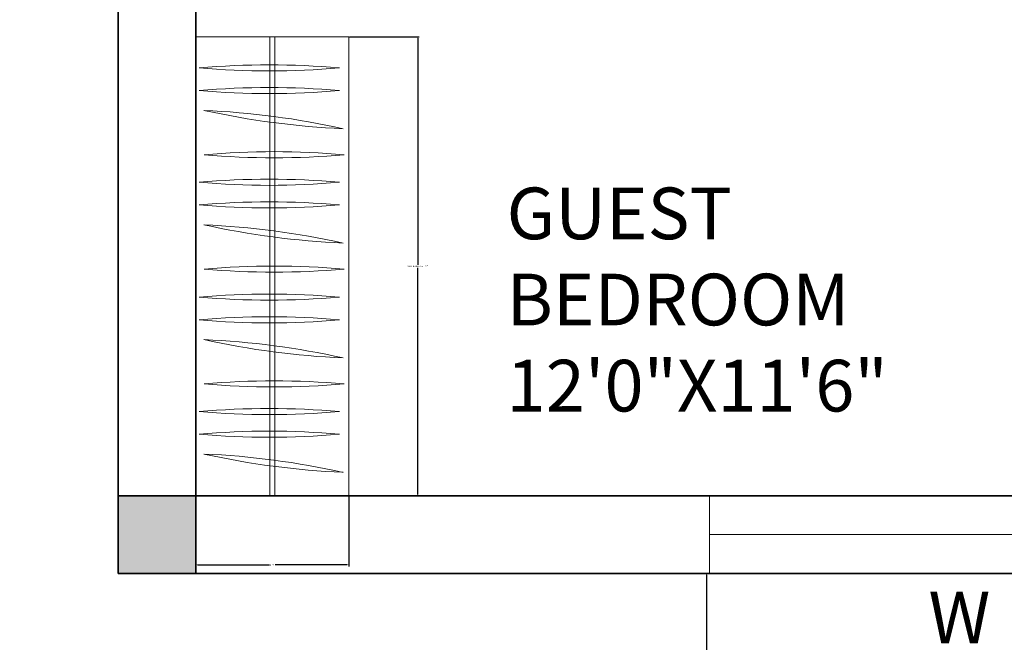
# Model space of a CAD drawing. Units: inches. Extents: x -36302355 to 648, y -221479757 to 75.
# Tile 30 of 37: x 227 to 341, y -139 to -67. Entities that reach past the tile are written whole.
import ezdxf

# ---------------------------------------------------------------- set-up
doc = ezdxf.new("R2010")
doc.units = ezdxf.units.IN
doc.header["$MEASUREMENT"] = 0
for name, color, linetype, lineweight in [('A-ANNO-DIMS', 2, 'Continuous', 18), ('A-ANNO-IDEN', 7, 'Continuous', 18), ('A-AREA-IDEN', 7, 'Continuous', 18), ('A-COLS-PATT', 242, 'Continuous', 13), ('A-FURN', 8, 'Continuous', 13), ('A-GLAZ', 142, 'Continuous', 18), ('A-WALL', 7, 'Continuous', 35)]:
    doc.layers.add(name, color=color, linetype=linetype, lineweight=lineweight)
doc.styles.get("Standard").update_dxf_attribs({"font": 'arial.ttf'})
doc.dimstyles.get("Standard").update_dxf_attribs({"dimtxt": 0.18, "dimasz": 0.18, "dimexe": 0.18, "dimexo": 0.0625, "dimgap": 0.09, "dimtad": 0, "dimtih": 1, "dimtoh": 1, "dimdec": 0, "dimzin": 0, "dimdsep": 46, "dimlunit": 3, "dimtxsty": 'Standard', "dimcen": 0.09, "dimadec": 0, "dimazin": 0, "dimtfac": 1, "dimtdec": 0, "dimtofl": 0, "dimtmove": 0, "dimatfit": 3, "dimfxl": 1, "dimtolj": 1, "dimtzin": 0, "dimarcsym": 0})

# ---------------------------------------------------------------- blocks, each defined once
blk = doc.blocks.new('*D1')
at = {"layer": 'A-ANNO-DIMS', "color": 0, "lineweight": -2, "transparency": 16777216}
for p, q in [((310.09, -131.02), (306.3, -131.02)), ((306.48, -131.2), (306.48, -145.86)), ((306.48, -166.84), (306.48, -152.17)), ((310.09, -167.02), (306.3, -167.02))]:
    blk.add_line(p, q, dxfattribs=at)
at = {"layer": 'A-ANNO-DIMS', "color": 0, "transparency": 16777216}
for points in [[(306.45, -131.2), (306.51, -131.2), (306.48, -131.02)], [(306.45, -166.84), (306.51, -166.84), (306.48, -167.02)]]:
    blk.add_solid(points, dxfattribs=at)
at = {"layer": 'Defpoints', "color": 0, "transparency": 16777216}
for p in [(310.15, -131.02), (306.48, -167.02), (310.15, -167.02)]:
    blk.add_point(p, dxfattribs=at)
at = {"layer": 'A-ANNO-DIMS', "color": 0, "transparency": 16777216, "insert": (306.48, -149.02), "char_height": 6, "attachment_point": 5}
blk.add_mtext("\\A1;3'", dxfattribs=at)
blk = doc.blocks.new('WARDROBE-HANGING')
for p, q in [((0, 0), (0, 53.32)), ((17.77, 53.32), (0, 53.32)), ((8.59, 0), (8.59, 53.32)), ((9.18, 0), (9.18, 53.32)), ((17.77, 0), (17.77, 53.32)), ((17.77, 0), (0, 0))]:
    blk.add_line(p, q)
for centre, start, end in [((8.53, -43.46), 85.0028, 94.9972), ((8.53, 142.85), 265.0028, 274.9972), ((8.53, -46.09), 85.0028, 94.9972), ((8.53, 140.22), 265.0028, 274.9972), ((21.18, 136.06), 257.508, 267.5023), ((-3.12, -48.66), 77.508, 87.5023), ((9.1, -53.54), 85.0028, 94.9972), ((9.1, 132.77), 265.0028, 274.9972), ((8.53, -56.74), 85.0028, 94.9972), ((8.53, 129.57), 265.0028, 274.9972), ((8.53, -59.37), 85.0028, 94.9972), ((8.53, 126.94), 265.0028, 274.9972), ((21.18, 122.78), 257.508, 267.5023), ((-3.12, -61.94), 77.508, 87.5023), ((9.1, -66.82), 85.0028, 94.9972), ((9.1, 119.49), 265.0028, 274.9972), ((8.53, -70.07), 85.0028, 94.9972), ((8.53, 116.24), 265.0028, 274.9972), ((8.53, -72.71), 85.0028, 94.9972), ((8.53, 113.6), 265.0028, 274.9972), ((-3.12, -75.27), 77.508, 87.5023), ((21.18, 109.44), 257.508, 267.5023), ((9.1, -80.15), 85.0028, 94.9972), ((9.1, 106.16), 265.0028, 274.9972), ((8.53, -83.36), 85.0028, 94.9972), ((8.53, 102.95), 265.0028, 274.9972), ((8.53, -85.99), 85.0028, 94.9972), ((8.53, 100.32), 265.0028, 274.9972), ((-3.12, -88.56), 77.508, 87.5023), ((21.18, 96.16), 257.508, 267.5023)]:
    blk.add_arc(centre, 93.51, start, end)
blk = doc.blocks.new('WIN-60')
for p, q in [((60, 9), (0, 9)), ((0, 9), (0, 0)), ((60, 0), (60, 9)), ((0, 4.5), (60, 4.5)), ((0, 0), (60, 0))]:
    blk.add_line(p, q)
blk = doc.blocks.new('*D43')
at = {"layer": 'A-ANNO-DIMS', "color": 0, "lineweight": -2, "transparency": 16777216}
for p, q in [((265.03, -68.7), (273.15, -68.7)), ((272.97, -68.88), (272.97, -95.18)), ((272.97, -121.84), (272.97, -95.54)), ((265.03, -122.02), (273.15, -122.02))]:
    blk.add_line(p, q, dxfattribs=at)
at = {"layer": 'A-ANNO-DIMS', "color": 0, "transparency": 16777216}
for points in [[(272.94, -68.88), (273, -68.88), (272.97, -68.7)], [(272.94, -121.84), (273, -121.84), (272.97, -122.02)]]:
    blk.add_solid(points, dxfattribs=at)
at = {"layer": 'Defpoints', "color": 0, "transparency": 16777216}
for p in [(264.97, -68.7), (272.97, -68.7), (264.97, -122.02)]:
    blk.add_point(p, dxfattribs=at)
at = {"layer": 'A-ANNO-DIMS', "color": 0, "transparency": 16777216, "insert": (272.97, -95.36), "char_height": 0.18, "attachment_point": 5}
blk.add_mtext('\\A1;WARDROBE 4\'-5 1/2"', dxfattribs=at)
blk = doc.blocks.new('*D44')
at = {"layer": 'A-ANNO-DIMS', "color": 0, "lineweight": -2, "transparency": 16777216}
for p, q in [((247.2, -122.08), (247.2, -130.2)), ((264.97, -122.08), (264.97, -130.2)), ((247.38, -130.02), (255.76, -130.02)), ((264.79, -130.02), (256.4, -130.02))]:
    blk.add_line(p, q, dxfattribs=at)
at = {"layer": 'A-ANNO-DIMS', "color": 0, "transparency": 16777216}
for points in [[(247.38, -129.99), (247.38, -130.05), (247.2, -130.02)], [(264.79, -129.99), (264.79, -130.05), (264.97, -130.02)]]:
    blk.add_solid(points, dxfattribs=at)
at = {"layer": 'Defpoints', "color": 0, "transparency": 16777216}
for p in [(247.2, -122.02), (264.97, -122.02), (264.97, -130.02)]:
    blk.add_point(p, dxfattribs=at)
at = {"layer": 'A-ANNO-DIMS', "color": 0, "transparency": 16777216, "insert": (256.08, -130.02), "char_height": 0.18, "attachment_point": 5}
blk.add_mtext('\\A1;1\'-6"', dxfattribs=at)

msp = doc.modelspace()

# ---------------------------------------------------------------- hatches: boundary and pattern name
at = {"layer": 'A-COLS-PATT'}
h = msp.add_hatch(color=256, dxfattribs=at)
h.dxf.hatch_style = 1
h.paths.add_polyline_path([(145.2, 24.98), (145.2, 15.98), (154.2, 15.98), (154.2, 24.98)])
h.paths.add_polyline_path([(247.2, 15.98), (247.2, 24.98), (238.2, 24.98), (238.2, 15.98)])
h.paths.add_polyline_path([(387.64, 15.98), (395.7, 15.98), (395.7, 24.98), (387.64, 24.98)])
h.paths.add_polyline_path([(451.26, 24.98), (443.7, 24.98), (443.7, 15.98), (451.26, 15.98)])
h.paths.add_polyline_path([(596.2, 15.98), (605.2, 15.98), (605.2, 24.98), (596.2, 24.98)])
h.paths.add_polyline_path([(238.2, -122.02), (238.2, -131.02), (247.2, -131.02), (247.2, -122.02)])
h.paths.add_polyline_path([(395.7, -122.02), (387.46, -122.02), (387.46, -131.02), (395.7, -131.02)])
h.paths.add_polyline_path([(448.2, -131.02), (453.73, -131.02), (453.73, -122.02), (443.7, -122.02), (443.7, -131.02)])
h.paths.add_polyline_path([(596.2, -131.02), (605.2, -131.02), (605.2, -122.02), (596.2, -122.02)])
h.paths.add_polyline_path([(145.2, -176.97), (154.2, -176.97), (154.2, -167.02), (145.2, -167.02)])
h.paths.add_polyline_path([(314.2, -176.97), (323.2, -176.97), (323.2, -167.02), (314.2, -167.02)])
h.paths.add_polyline_path([(154.2, -314.02), (154.2, -309.52), (145.2, -309.52), (145.2, -314.02)])
h.paths.add_polyline_path([(314.2, -309.52), (314.2, -318.52), (323.2, -318.52), (323.2, -309.52)])
h.paths.add_polyline_path([(448.2, -277.02), (443.7, -277.02), (443.7, -286.02), (448.2, -286.02)])
h.paths.add_polyline_path([(283.2, -370.02), (274.2, -370.02), (274.2, -379.02), (283.2, -379.02), (283.2, -374.52)])
h.paths.add_polyline_path([(154.2, -370.02), (145.2, -370.02), (145.2, -379.02), (154.2, -379.02)])
h.paths.add_polyline_path([(443.2, -374.52), (443.2, -379.02), (452.2, -379.02), (452.2, -374.52)])
h.paths.add_polyline_path([(145.2, -580.02), (154.2, -580.02), (154.2, -571.02), (145.2, -571.02)])
h.paths.add_polyline_path([(274.2, -571.02), (274.2, -580.02), (283.2, -580.02), (283.2, -571.02)])
h.paths.add_polyline_path([(443.2, -580.02), (452.2, -580.02), (452.2, -571.02), (443.2, -571.02)])

# ---------------------------------------------------------------- linework, layer by layer
at = {"layer": 'A-WALL'}
for p, q in [((238.2, 24.98), (238.2, -131.02)), ((247.2, 24.98), (247.2, -131.02)), ((238.2, -122.02), (395.7, -122.02)), ((238.2, -131.02), (395.7, -131.02))]:
    msp.add_line(p, q, dxfattribs=at)

# ---------------------------------------------------------------- block references
at = {"layer": 'A-FURN'}
msp.add_blockref('WARDROBE-HANGING', (247.2, -122.02), dxfattribs=at)
at = {"layer": 'A-GLAZ'}
msp.add_blockref('WIN-60', (306.86, -131.02), dxfattribs=at)

# ---------------------------------------------------------------- texts
at = {"layer": 'A-ANNO-IDEN', "insert": (332.27, -133.13), "char_height": 6, "attachment_point": 1}
msp.add_mtext_dynamic_manual_height_columns('W', width=2.1009, gutter_width=1, heights=[0], dxfattribs=at)
at = {"layer": 'A-AREA-IDEN', "insert": (283.29, -86.22), "char_height": 6, "attachment_point": 1}
msp.add_mtext('GUEST\\PBEDROOM\\P12\'0"X11\'6"', dxfattribs=at)

# ---------------------------------------------------------------- dimensions: what is measured, and where the dimension line sits
at = {"layer": 'A-ANNO-DIMS'}
dim = msp.add_linear_dim(base=(272.97, -68.7), p1=(264.97, -122.02), p2=(264.97, -68.7), angle=90, text='WARDROBE <>', dimstyle='Standard', override={"dimdec": 1, "dimlfac": 1, "dimrnd": 0, "dimzin": 1, "dimdsep": 46, "dimlunit": 4, "dimfrac": 2}, dxfattribs=at)
dim.commit()
dim.dimension.update_dxf_attribs({"geometry": '*D43', "text_midpoint": (272.97, -95.36)})
dim = msp.add_linear_dim(base=(264.97, -130.02), p1=(247.2, -122.02), p2=(264.97, -122.02), dimstyle='Standard', override={"dimdec": 1, "dimlfac": 1, "dimrnd": 0, "dimzin": 1, "dimdsep": 46, "dimlunit": 4, "dimfrac": 2}, dxfattribs=at)
dim.commit()
dim.dimension.update_dxf_attribs({"geometry": '*D44', "text_midpoint": (256.08, -130.02)})
dim = msp.add_linear_dim(base=(306.48, -167.02), p1=(310.15, -131.02), p2=(310.15, -167.02), angle=90, dimstyle='Standard', override={"dimtxt": 6, "dimclrd": 0, "dimclre": 0, "dimclrt": 0}, dxfattribs=at)
dim.commit()
dim.dimension.update_dxf_attribs({"geometry": '*D1', "text_midpoint": (306.48, -149.02)})

doc.saveas('drawing.dxf')
